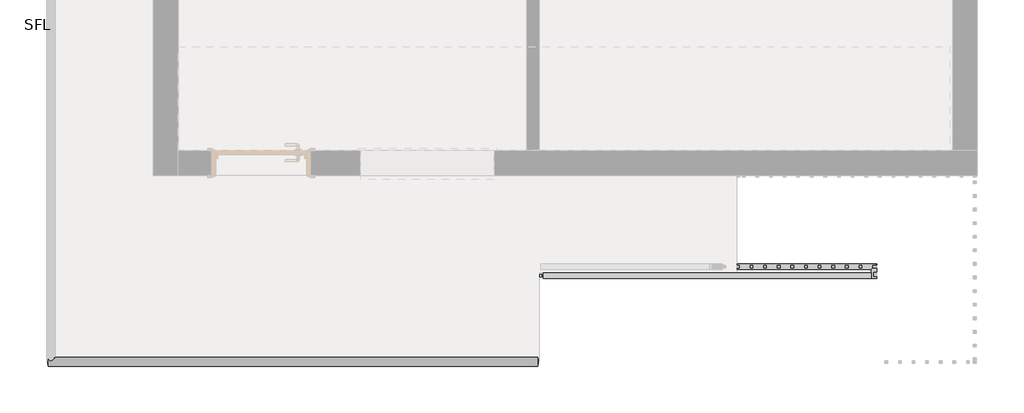
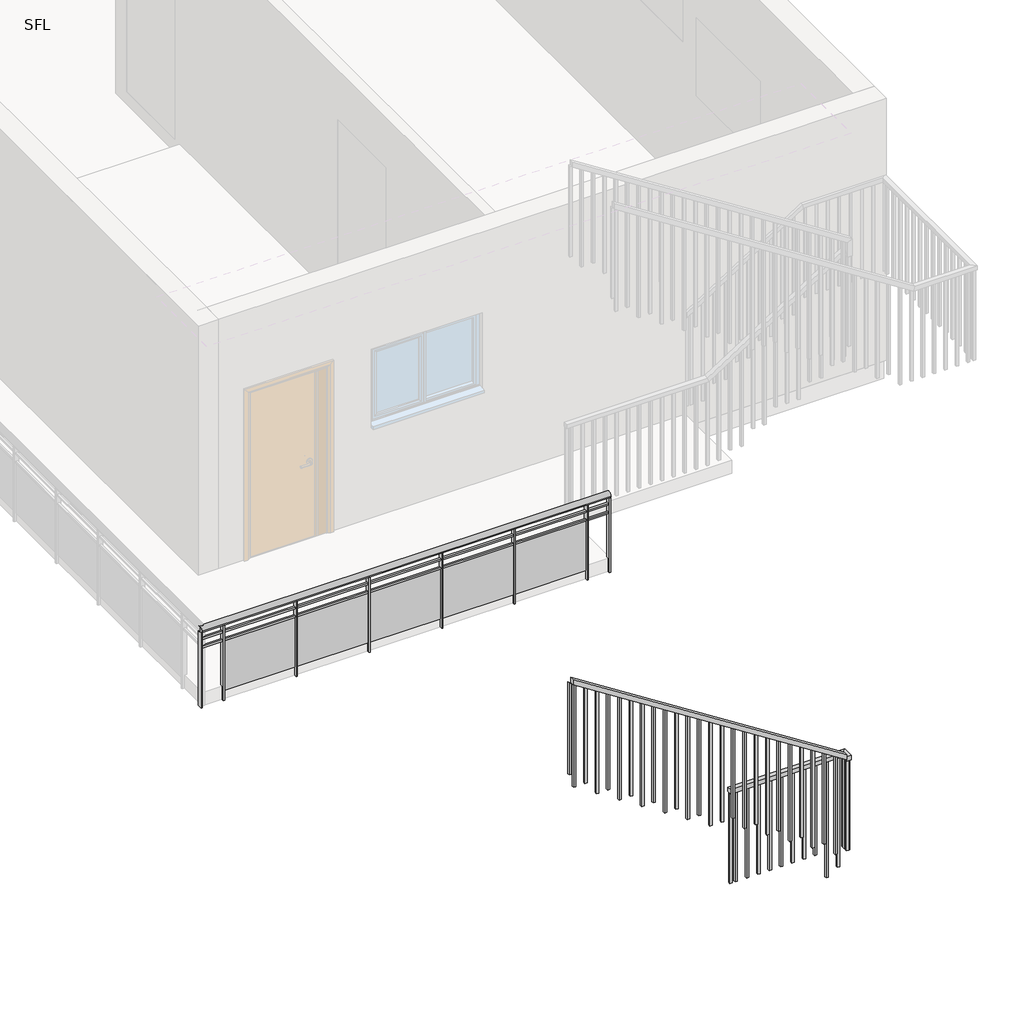
# One storey, part 2 of 4: 3 railings.
"""IFC4 building model written with IfcOpenShell, lengths in millimetres."""

from ifc_helpers import new_model, si_unit, point, frame, origin, place, context, project, spatial, polyline, ellipse_curve, trimmed, outline, extrude, faceted_brep, element, save
from ifc_brep_helpers import plane_surface, extruded_surface, advanced_brep

model = new_model("IFC4")

# Units and contexts
model_context = context("Model", 3, world=origin())
ifc_project = project(units=[si_unit("LENGTHUNIT", "METRE", prefix="MILLI")], contexts=[model_context])

# Site, building, storey
site = spatial("IfcSite", under=ifc_project)
building = spatial("IfcBuilding", under=site)
storey = spatial("IfcBuildingStorey", under=building, Name="SFL", Elevation=6583.68)

# Railings
placement = place(None, origin())
element("IfcRailing", 1, ObjectType="1100mm", at=placement, inside=storey, context=model_context, shape_type="SolidModel", body=[
    faceted_brep([(-10457.8773536, -11114.0601959, 4838.88), (-10457.8773536, -11114.0601959, 4779.5164137), (-10457.8773536, -11164.0601959, 4779.5164137), (-10457.8773536, -11164.0601959, 4838.88), (-7447.5340108, -11114.0601959, 2912.2269781), (-7447.5340108, -11164.0601959, 2912.2269781), (-7447.5340108, -11164.0601959, 2852.8633918), (-7447.5340108, -11114.0601959, 2852.8633918)], [[[0, 1, 2, 3]], [[4, 5, 6, 7]], [[1, 0, 4, 7]], [[2, 1, 7, 6]], [[3, 2, 6, 5]], [[0, 3, 5, 4]]]),
    faceted_brep([(-7447.5340108, -11164.0601959, 2888.16), (-7447.5340108, -11164.0601959, 2838.16), (-7397.5340108, -11164.0601959, 2838.16), (-7397.5340108, -11164.0601959, 2888.16), (-7447.5340108, -11083.3255223, 2888.16), (-7447.5340108, -11083.3255223, 2838.16), (-7397.5340108, -11033.3255223, 2838.16), (-7397.5340108, -11033.3255223, 2888.16), (-8680.149573, -11083.3255223, 2888.16), (-8680.149573, -11033.3255223, 2888.16), (-8680.149573, -11033.3255223, 2838.16), (-8680.149573, -11083.3255223, 2838.16)], [[[0, 1, 2, 3]], [[1, 0, 4, 5]], [[2, 1, 5, 6]], [[3, 2, 6, 7]], [[0, 3, 7, 4]], [[8, 9, 10, 11]], [[5, 4, 8, 11]], [[6, 5, 11, 10]], [[7, 6, 10, 9]], [[4, 7, 9, 8]]]),
    extrude(outline(polyline([(-8597.5340108, -11045.8255223), (-8597.5340108, -11070.8255223), (-8622.5340108, -11070.8255223), (-8622.5340108, -11045.8255223), (-8597.5340108, -11045.8255223)])), frame((0.0, 0.0, 1788.16), z_axis=(0.0, 0.0, 1.0), x_axis=(1.0, 0.0, 0.0)), (0.0, 0.0, 1.0), 1050.0),
    extrude(outline(polyline([(-8472.5340108, -11045.8255223), (-8472.5340108, -11070.8255223), (-8497.5340108, -11070.8255223), (-8497.5340108, -11045.8255223), (-8472.5340108, -11045.8255223)])), frame((0.0, 0.0, 1788.16), z_axis=(0.0, 0.0, 1.0), x_axis=(1.0, 0.0, 0.0)), (0.0, 0.0, 1.0), 1050.0),
    extrude(outline(polyline([(-8347.5340108, -11045.8255223), (-8347.5340108, -11070.8255223), (-8372.5340108, -11070.8255223), (-8372.5340108, -11045.8255223), (-8347.5340108, -11045.8255223)])), frame((0.0, 0.0, 1788.16), z_axis=(0.0, 0.0, 1.0), x_axis=(1.0, 0.0, 0.0)), (0.0, 0.0, 1.0), 1050.0),
    extrude(outline(polyline([(-8222.5340108, -11045.8255223), (-8222.5340108, -11070.8255223), (-8247.5340108, -11070.8255223), (-8247.5340108, -11045.8255223), (-8222.5340108, -11045.8255223)])), frame((0.0, 0.0, 1788.16), z_axis=(0.0, 0.0, 1.0), x_axis=(1.0, 0.0, 0.0)), (0.0, 0.0, 1.0), 1050.0),
    extrude(outline(polyline([(-8097.5340108, -11045.8255223), (-8097.5340108, -11070.8255223), (-8122.5340108, -11070.8255223), (-8122.5340108, -11045.8255223), (-8097.5340108, -11045.8255223)])), frame((0.0, 0.0, 1788.16), z_axis=(0.0, 0.0, 1.0), x_axis=(1.0, 0.0, 0.0)), (0.0, 0.0, 1.0), 1050.0),
    extrude(outline(polyline([(-7972.5340108, -11045.8255223), (-7972.5340108, -11070.8255223), (-7997.5340108, -11070.8255223), (-7997.5340108, -11045.8255223), (-7972.5340108, -11045.8255223)])), frame((0.0, 0.0, 1788.16), z_axis=(0.0, 0.0, 1.0), x_axis=(1.0, 0.0, 0.0)), (0.0, 0.0, 1.0), 1050.0),
    extrude(outline(polyline([(-7847.5340108, -11045.8255223), (-7847.5340108, -11070.8255223), (-7872.5340108, -11070.8255223), (-7872.5340108, -11045.8255223), (-7847.5340108, -11045.8255223)])), frame((0.0, 0.0, 1788.16), z_axis=(0.0, 0.0, 1.0), x_axis=(1.0, 0.0, 0.0)), (0.0, 0.0, 1.0), 1050.0),
    extrude(outline(polyline([(-7722.5340108, -11045.8255223), (-7722.5340108, -11070.8255223), (-7747.5340108, -11070.8255223), (-7747.5340108, -11045.8255223), (-7722.5340108, -11045.8255223)])), frame((0.0, 0.0, 1788.16), z_axis=(0.0, 0.0, 1.0), x_axis=(1.0, 0.0, 0.0)), (0.0, 0.0, 1.0), 1050.0),
    extrude(outline(polyline([(-7597.5340108, -11045.8255223), (-7597.5340108, -11070.8255223), (-7622.5340108, -11070.8255223), (-7622.5340108, -11045.8255223), (-7597.5340108, -11045.8255223)])), frame((0.0, 0.0, 1484.4784954), z_axis=(0.0, 0.0, 1.0), x_axis=(1.0, 0.0, 0.0)), (0.0, 0.0, 1.0), 1353.6815046),
    extrude(outline(polyline([(-7472.5340108, -11045.8255223), (-7472.5340108, -11070.8255223), (-7497.5340108, -11070.8255223), (-7497.5340108, -11045.8255223), (-7472.5340108, -11045.8255223)])), frame((0.0, 0.0, 1564.4608651), z_axis=(0.0, 0.0, 1.0), x_axis=(1.0, 0.0, 0.0)), (0.0, 0.0, 1.0), 1273.6991349),
    extrude(outline(polyline([(-7410.0340108, -11089.0601959), (-7435.0340108, -11089.0601959), (-7435.0340108, -11064.0601959), (-7410.0340108, -11064.0601959), (-7410.0340108, -11089.0601959)])), frame((0.0, 0.0, 1770.6), z_axis=(0.0, 0.0, 1.0), x_axis=(1.0, 0.0, 0.0)), (0.0, 0.0, 1.0), 1067.56),
    extrude(outline(polyline([(2851.8393741, -7445.9340108), (1788.16, -7445.9340108), (1788.16, -7420.9340108), (2835.8390977, -7420.9340108), (2851.8393741, -7445.9340108)])), frame((0.0, -11151.5601959, 0.0), z_axis=(0.0, 1.0, 0.0), x_axis=(0.0, 0.0, 1.0)), (0.0, 0.0, 1.0), 25.0),
    extrude(outline(polyline([(2931.8407561, -7570.9340108), (1788.16, -7570.9340108), (1788.16, -7545.9340108), (2915.8404797, -7545.9340108), (2931.8407561, -7570.9340108)])), frame((0.0, -11151.5601959, 0.0), z_axis=(0.0, 1.0, 0.0), x_axis=(0.0, 0.0, 1.0)), (0.0, 0.0, 1.0), 25.0),
    extrude(outline(polyline([(3011.8421381, -7695.9340108), (1950.72, -7695.9340108), (1950.72, -7670.9340108), (2995.8418617, -7670.9340108), (3011.8421381, -7695.9340108)])), frame((0.0, -11151.5601959, 0.0), z_axis=(0.0, 1.0, 0.0), x_axis=(0.0, 0.0, 1.0)), (0.0, 0.0, 1.0), 25.0),
    extrude(outline(polyline([(3091.8435201, -7820.9340108), (1950.72, -7820.9340108), (1950.72, -7795.9340108), (3075.8432437, -7795.9340108), (3091.8435201, -7820.9340108)])), frame((0.0, -11151.5601959, 0.0), z_axis=(0.0, 1.0, 0.0), x_axis=(0.0, 0.0, 1.0)), (0.0, 0.0, 1.0), 25.0),
    extrude(outline(polyline([(3171.8449021, -7945.9340108), (2113.28, -7945.9340108), (2113.28, -7920.9340108), (3155.8446257, -7920.9340108), (3171.8449021, -7945.9340108)])), frame((0.0, -11151.5601959, 0.0), z_axis=(0.0, 1.0, 0.0), x_axis=(0.0, 0.0, 1.0)), (0.0, 0.0, 1.0), 25.0),
    extrude(outline(polyline([(3251.8462841, -8070.9340108), (2113.28, -8070.9340108), (2113.28, -8045.9340108), (3235.8460077, -8045.9340108), (3251.8462841, -8070.9340108)])), frame((0.0, -11151.5601959, 0.0), z_axis=(0.0, 1.0, 0.0), x_axis=(0.0, 0.0, 1.0)), (0.0, 0.0, 1.0), 25.0),
    extrude(outline(polyline([(3331.8476661, -8195.9340108), (2275.84, -8195.9340108), (2275.84, -8170.9340108), (3315.8473897, -8170.9340108), (3331.8476661, -8195.9340108)])), frame((0.0, -11151.5601959, 0.0), z_axis=(0.0, 1.0, 0.0), x_axis=(0.0, 0.0, 1.0)), (0.0, 0.0, 1.0), 25.0),
    extrude(outline(polyline([(3411.8490481, -8320.9340108), (2275.84, -8320.9340108), (2275.84, -8295.9340108), (3395.8487717, -8295.9340108), (3411.8490481, -8320.9340108)])), frame((0.0, -11151.5601959, 0.0), z_axis=(0.0, 1.0, 0.0), x_axis=(0.0, 0.0, 1.0)), (0.0, 0.0, 1.0), 25.0),
    extrude(outline(polyline([(3491.8504301, -8445.9340108), (2438.4, -8445.9340108), (2438.4, -8420.9340108), (3475.8501537, -8420.9340108), (3491.8504301, -8445.9340108)])), frame((0.0, -11151.5601959, 0.0), z_axis=(0.0, 1.0, 0.0), x_axis=(0.0, 0.0, 1.0)), (0.0, 0.0, 1.0), 25.0),
    extrude(outline(polyline([(3571.8518121, -8570.9340108), (2438.4, -8570.9340108), (2438.4, -8545.9340108), (3555.8515357, -8545.9340108), (3571.8518121, -8570.9340108)])), frame((0.0, -11151.5601959, 0.0), z_axis=(0.0, 1.0, 0.0), x_axis=(0.0, 0.0, 1.0)), (0.0, 0.0, 1.0), 25.0),
    extrude(outline(polyline([(3651.8531942, -8695.9340108), (2600.96, -8695.9340108), (2600.96, -8670.9340108), (3635.8529178, -8670.9340108), (3651.8531942, -8695.9340108)])), frame((0.0, -11151.5601959, 0.0), z_axis=(0.0, 1.0, 0.0), x_axis=(0.0, 0.0, 1.0)), (0.0, 0.0, 1.0), 25.0),
    extrude(outline(polyline([(3731.8545762, -8820.9340108), (2600.96, -8820.9340108), (2600.96, -8795.9340108), (3715.8542998, -8795.9340108), (3731.8545762, -8820.9340108)])), frame((0.0, -11151.5601959, 0.0), z_axis=(0.0, 1.0, 0.0), x_axis=(0.0, 0.0, 1.0)), (0.0, 0.0, 1.0), 25.0),
    extrude(outline(polyline([(3811.8559582, -8945.9340108), (2600.96, -8945.9340108), (2600.96, -8920.9340108), (3795.8556818, -8920.9340108), (3811.8559582, -8945.9340108)])), frame((0.0, -11151.5601959, 0.0), z_axis=(0.0, 1.0, 0.0), x_axis=(0.0, 0.0, 1.0)), (0.0, 0.0, 1.0), 25.0),
    extrude(outline(polyline([(3891.8573402, -9070.9340108), (2763.52, -9070.9340108), (2763.52, -9045.9340108), (3875.8570638, -9045.9340108), (3891.8573402, -9070.9340108)])), frame((0.0, -11151.5601959, 0.0), z_axis=(0.0, 1.0, 0.0), x_axis=(0.0, 0.0, 1.0)), (0.0, 0.0, 1.0), 25.0),
    extrude(outline(polyline([(3971.8587222, -9195.9340108), (2763.52, -9195.9340108), (2763.52, -9170.9340108), (3955.8584458, -9170.9340108), (3971.8587222, -9195.9340108)])), frame((0.0, -11151.5601959, 0.0), z_axis=(0.0, 1.0, 0.0), x_axis=(0.0, 0.0, 1.0)), (0.0, 0.0, 1.0), 25.0),
    extrude(outline(polyline([(4051.8601042, -9320.9340108), (2926.08, -9320.9340108), (2926.08, -9295.9340108), (4035.8598278, -9295.9340108), (4051.8601042, -9320.9340108)])), frame((0.0, -11151.5601959, 0.0), z_axis=(0.0, 1.0, 0.0), x_axis=(0.0, 0.0, 1.0)), (0.0, 0.0, 1.0), 25.0),
    extrude(outline(polyline([(4131.8614862, -9445.9340108), (2926.08, -9445.9340108), (2926.08, -9420.9340108), (4115.8612098, -9420.9340108), (4131.8614862, -9445.9340108)])), frame((0.0, -11151.5601959, 0.0), z_axis=(0.0, 1.0, 0.0), x_axis=(0.0, 0.0, 1.0)), (0.0, 0.0, 1.0), 25.0),
    extrude(outline(polyline([(4211.8628682, -9570.9340108), (3088.64, -9570.9340108), (3088.64, -9545.9340108), (4195.8625918, -9545.9340108), (4211.8628682, -9570.9340108)])), frame((0.0, -11151.5601959, 0.0), z_axis=(0.0, 1.0, 0.0), x_axis=(0.0, 0.0, 1.0)), (0.0, 0.0, 1.0), 25.0),
    extrude(outline(polyline([(4291.8642502, -9695.9340108), (3088.64, -9695.9340108), (3088.64, -9670.9340108), (4275.8639738, -9670.9340108), (4291.8642502, -9695.9340108)])), frame((0.0, -11151.5601959, 0.0), z_axis=(0.0, 1.0, 0.0), x_axis=(0.0, 0.0, 1.0)), (0.0, 0.0, 1.0), 25.0),
    extrude(outline(polyline([(4371.8656322, -9820.9340108), (3251.2, -9820.9340108), (3251.2, -9795.9340108), (4355.8653558, -9795.9340108), (4371.8656322, -9820.9340108)])), frame((0.0, -11151.5601959, 0.0), z_axis=(0.0, 1.0, 0.0), x_axis=(0.0, 0.0, 1.0)), (0.0, 0.0, 1.0), 25.0),
    extrude(outline(polyline([(4451.8670143, -9945.9340108), (3251.2, -9945.9340108), (3251.2, -9920.9340108), (4435.8667379, -9920.9340108), (4451.8670143, -9945.9340108)])), frame((0.0, -11151.5601959, 0.0), z_axis=(0.0, 1.0, 0.0), x_axis=(0.0, 0.0, 1.0)), (0.0, 0.0, 1.0), 25.0),
    extrude(outline(polyline([(4531.8683963, -10070.9340108), (3413.76, -10070.9340108), (3413.76, -10045.9340108), (4515.8681199, -10045.9340108), (4531.8683963, -10070.9340108)])), frame((0.0, -11151.5601959, 0.0), z_axis=(0.0, 1.0, 0.0), x_axis=(0.0, 0.0, 1.0)), (0.0, 0.0, 1.0), 25.0),
    extrude(outline(polyline([(4611.8697783, -10195.9340108), (3413.76, -10195.9340108), (3413.76, -10170.9340108), (4595.8695019, -10170.9340108), (4611.8697783, -10195.9340108)])), frame((0.0, -11151.5601959, 0.0), z_axis=(0.0, 1.0, 0.0), x_axis=(0.0, 0.0, 1.0)), (0.0, 0.0, 1.0), 25.0),
    extrude(outline(polyline([(4691.8711603, -10320.9340108), (3576.32, -10320.9340108), (3576.32, -10295.9340108), (4675.8708839, -10295.9340108), (4691.8711603, -10320.9340108)])), frame((0.0, -11151.5601959, 0.0), z_axis=(0.0, 1.0, 0.0), x_axis=(0.0, 0.0, 1.0)), (0.0, 0.0, 1.0), 25.0),
    extrude(outline(polyline([(4771.8725423, -10445.9340108), (3576.32, -10445.9340108), (3576.32, -10420.9340108), (4755.8722659, -10420.9340108), (4771.8725423, -10445.9340108)])), frame((0.0, -11151.5601959, 0.0), z_axis=(0.0, 1.0, 0.0), x_axis=(0.0, 0.0, 1.0)), (0.0, 0.0, 1.0), 25.0),
    extrude(outline(polyline([(-7410.0340108, -11070.8255223), (-7435.0340108, -11070.8255223), (-7435.0340108, -11045.8255223), (-7410.0340108, -11045.8255223), (-7410.0340108, -11070.8255223)])), frame((0.0, 0.0, 1770.6), z_axis=(0.0, 0.0, 1.0), x_axis=(1.0, 0.0, 0.0)), (0.0, 0.0, 1.0), 1067.56),
    extrude(outline(polyline([(2844.8632536, -7435.0340108), (1788.16, -7435.0340108), (1788.16, -7410.0340108), (2828.8629772, -7410.0340108), (2844.8632536, -7435.0340108)])), frame((0.0, -11151.5601959, 0.0), z_axis=(0.0, 1.0, 0.0), x_axis=(0.0, 0.0, 1.0)), (0.0, 0.0, 1.0), 25.0),
    extrude(outline(polyline([(-8655.149573, -11045.8255223), (-8655.149573, -11070.8255223), (-8680.149573, -11070.8255223), (-8680.149573, -11045.8255223), (-8655.149573, -11045.8255223)])), frame((0.0, 0.0, 1788.16), z_axis=(0.0, 0.0, 1.0), x_axis=(1.0, 0.0, 0.0)), (0.0, 0.0, 1.0), 1050.0),
    extrude(outline(polyline([(4803.8730951, -10495.9340108), (3738.88, -10495.9340108), (3738.88, -10470.9340108), (4787.8728187, -10470.9340108), (4803.8730951, -10495.9340108)])), frame((0.0, -11151.5601959, 0.0), z_axis=(0.0, 1.0, 0.0), x_axis=(0.0, 0.0, 1.0)), (0.0, 0.0, 1.0), 25.0),
])
element("IfcRailing", 2, ObjectType="1100mm", at=placement, inside=storey, context=model_context, shape_type="SolidModel", body=[
    faceted_brep([(-10457.8773536, -11114.0601959, 4838.88), (-10457.8773536, -11114.0601959, 4779.5164137), (-10457.8773536, -11164.0601959, 4779.5164137), (-10457.8773536, -11164.0601959, 4838.88), (-7447.5340108, -11114.0601959, 2912.2269781), (-7447.5340108, -11164.0601959, 2912.2269781), (-7447.5340108, -11164.0601959, 2852.8633918), (-7447.5340108, -11114.0601959, 2852.8633918)], [[[0, 1, 2, 3]], [[4, 5, 6, 7]], [[1, 0, 4, 7]], [[2, 1, 7, 6]], [[3, 2, 6, 5]], [[0, 3, 5, 4]]]),
    faceted_brep([(-7447.5340108, -11164.0601959, 2888.16), (-7447.5340108, -11164.0601959, 2838.16), (-7397.5340108, -11164.0601959, 2838.16), (-7397.5340108, -11164.0601959, 2888.16), (-7447.5340108, -11083.3255223, 2888.16), (-7447.5340108, -11083.3255223, 2838.16), (-7397.5340108, -11033.3255223, 2838.16), (-7397.5340108, -11033.3255223, 2888.16), (-8680.149573, -11083.3255223, 2888.16), (-8680.149573, -11033.3255223, 2888.16), (-8680.149573, -11033.3255223, 2838.16), (-8680.149573, -11083.3255223, 2838.16)], [[[0, 1, 2, 3]], [[1, 0, 4, 5]], [[2, 1, 5, 6]], [[3, 2, 6, 7]], [[0, 3, 7, 4]], [[8, 9, 10, 11]], [[5, 4, 8, 11]], [[6, 5, 11, 10]], [[7, 6, 10, 9]], [[4, 7, 9, 8]]]),
    extrude(outline(polyline([(-8597.5340108, -11045.8255223), (-8597.5340108, -11070.8255223), (-8622.5340108, -11070.8255223), (-8622.5340108, -11045.8255223), (-8597.5340108, -11045.8255223)])), frame((0.0, 0.0, 1788.16), z_axis=(0.0, 0.0, 1.0), x_axis=(1.0, 0.0, 0.0)), (0.0, 0.0, 1.0), 1050.0),
    extrude(outline(polyline([(-8472.5340108, -11045.8255223), (-8472.5340108, -11070.8255223), (-8497.5340108, -11070.8255223), (-8497.5340108, -11045.8255223), (-8472.5340108, -11045.8255223)])), frame((0.0, 0.0, 1788.16), z_axis=(0.0, 0.0, 1.0), x_axis=(1.0, 0.0, 0.0)), (0.0, 0.0, 1.0), 1050.0),
    extrude(outline(polyline([(-8347.5340108, -11045.8255223), (-8347.5340108, -11070.8255223), (-8372.5340108, -11070.8255223), (-8372.5340108, -11045.8255223), (-8347.5340108, -11045.8255223)])), frame((0.0, 0.0, 1788.16), z_axis=(0.0, 0.0, 1.0), x_axis=(1.0, 0.0, 0.0)), (0.0, 0.0, 1.0), 1050.0),
    extrude(outline(polyline([(-8222.5340108, -11045.8255223), (-8222.5340108, -11070.8255223), (-8247.5340108, -11070.8255223), (-8247.5340108, -11045.8255223), (-8222.5340108, -11045.8255223)])), frame((0.0, 0.0, 1788.16), z_axis=(0.0, 0.0, 1.0), x_axis=(1.0, 0.0, 0.0)), (0.0, 0.0, 1.0), 1050.0),
    extrude(outline(polyline([(-8097.5340108, -11045.8255223), (-8097.5340108, -11070.8255223), (-8122.5340108, -11070.8255223), (-8122.5340108, -11045.8255223), (-8097.5340108, -11045.8255223)])), frame((0.0, 0.0, 1788.16), z_axis=(0.0, 0.0, 1.0), x_axis=(1.0, 0.0, 0.0)), (0.0, 0.0, 1.0), 1050.0),
    extrude(outline(polyline([(-7972.5340108, -11045.8255223), (-7972.5340108, -11070.8255223), (-7997.5340108, -11070.8255223), (-7997.5340108, -11045.8255223), (-7972.5340108, -11045.8255223)])), frame((0.0, 0.0, 1788.16), z_axis=(0.0, 0.0, 1.0), x_axis=(1.0, 0.0, 0.0)), (0.0, 0.0, 1.0), 1050.0),
    extrude(outline(polyline([(-7847.5340108, -11045.8255223), (-7847.5340108, -11070.8255223), (-7872.5340108, -11070.8255223), (-7872.5340108, -11045.8255223), (-7847.5340108, -11045.8255223)])), frame((0.0, 0.0, 1788.16), z_axis=(0.0, 0.0, 1.0), x_axis=(1.0, 0.0, 0.0)), (0.0, 0.0, 1.0), 1050.0),
    extrude(outline(polyline([(-7722.5340108, -11045.8255223), (-7722.5340108, -11070.8255223), (-7747.5340108, -11070.8255223), (-7747.5340108, -11045.8255223), (-7722.5340108, -11045.8255223)])), frame((0.0, 0.0, 1788.16), z_axis=(0.0, 0.0, 1.0), x_axis=(1.0, 0.0, 0.0)), (0.0, 0.0, 1.0), 1050.0),
    extrude(outline(polyline([(-7597.5340108, -11045.8255223), (-7597.5340108, -11070.8255223), (-7622.5340108, -11070.8255223), (-7622.5340108, -11045.8255223), (-7597.5340108, -11045.8255223)])), frame((0.0, 0.0, 1484.4784954), z_axis=(0.0, 0.0, 1.0), x_axis=(1.0, 0.0, 0.0)), (0.0, 0.0, 1.0), 1353.6815046),
    extrude(outline(polyline([(-7472.5340108, -11045.8255223), (-7472.5340108, -11070.8255223), (-7497.5340108, -11070.8255223), (-7497.5340108, -11045.8255223), (-7472.5340108, -11045.8255223)])), frame((0.0, 0.0, 1564.4608651), z_axis=(0.0, 0.0, 1.0), x_axis=(1.0, 0.0, 0.0)), (0.0, 0.0, 1.0), 1273.6991349),
    extrude(outline(polyline([(-7410.0340108, -11089.0601959), (-7435.0340108, -11089.0601959), (-7435.0340108, -11064.0601959), (-7410.0340108, -11064.0601959), (-7410.0340108, -11089.0601959)])), frame((0.0, 0.0, 1770.6), z_axis=(0.0, 0.0, 1.0), x_axis=(1.0, 0.0, 0.0)), (0.0, 0.0, 1.0), 1067.56),
    extrude(outline(polyline([(2851.8393741, -7445.9340108), (1788.16, -7445.9340108), (1788.16, -7420.9340108), (2835.8390977, -7420.9340108), (2851.8393741, -7445.9340108)])), frame((0.0, -11151.5601959, 0.0), z_axis=(0.0, 1.0, 0.0), x_axis=(0.0, 0.0, 1.0)), (0.0, 0.0, 1.0), 25.0),
    extrude(outline(polyline([(2931.8407561, -7570.9340108), (1788.16, -7570.9340108), (1788.16, -7545.9340108), (2915.8404797, -7545.9340108), (2931.8407561, -7570.9340108)])), frame((0.0, -11151.5601959, 0.0), z_axis=(0.0, 1.0, 0.0), x_axis=(0.0, 0.0, 1.0)), (0.0, 0.0, 1.0), 25.0),
    extrude(outline(polyline([(3011.8421381, -7695.9340108), (1950.72, -7695.9340108), (1950.72, -7670.9340108), (2995.8418617, -7670.9340108), (3011.8421381, -7695.9340108)])), frame((0.0, -11151.5601959, 0.0), z_axis=(0.0, 1.0, 0.0), x_axis=(0.0, 0.0, 1.0)), (0.0, 0.0, 1.0), 25.0),
    extrude(outline(polyline([(3091.8435201, -7820.9340108), (1950.72, -7820.9340108), (1950.72, -7795.9340108), (3075.8432437, -7795.9340108), (3091.8435201, -7820.9340108)])), frame((0.0, -11151.5601959, 0.0), z_axis=(0.0, 1.0, 0.0), x_axis=(0.0, 0.0, 1.0)), (0.0, 0.0, 1.0), 25.0),
    extrude(outline(polyline([(3171.8449021, -7945.9340108), (2113.28, -7945.9340108), (2113.28, -7920.9340108), (3155.8446257, -7920.9340108), (3171.8449021, -7945.9340108)])), frame((0.0, -11151.5601959, 0.0), z_axis=(0.0, 1.0, 0.0), x_axis=(0.0, 0.0, 1.0)), (0.0, 0.0, 1.0), 25.0),
    extrude(outline(polyline([(3251.8462841, -8070.9340108), (2113.28, -8070.9340108), (2113.28, -8045.9340108), (3235.8460077, -8045.9340108), (3251.8462841, -8070.9340108)])), frame((0.0, -11151.5601959, 0.0), z_axis=(0.0, 1.0, 0.0), x_axis=(0.0, 0.0, 1.0)), (0.0, 0.0, 1.0), 25.0),
    extrude(outline(polyline([(3331.8476661, -8195.9340108), (2275.84, -8195.9340108), (2275.84, -8170.9340108), (3315.8473897, -8170.9340108), (3331.8476661, -8195.9340108)])), frame((0.0, -11151.5601959, 0.0), z_axis=(0.0, 1.0, 0.0), x_axis=(0.0, 0.0, 1.0)), (0.0, 0.0, 1.0), 25.0),
    extrude(outline(polyline([(3411.8490481, -8320.9340108), (2275.84, -8320.9340108), (2275.84, -8295.9340108), (3395.8487717, -8295.9340108), (3411.8490481, -8320.9340108)])), frame((0.0, -11151.5601959, 0.0), z_axis=(0.0, 1.0, 0.0), x_axis=(0.0, 0.0, 1.0)), (0.0, 0.0, 1.0), 25.0),
    extrude(outline(polyline([(3491.8504301, -8445.9340108), (2438.4, -8445.9340108), (2438.4, -8420.9340108), (3475.8501537, -8420.9340108), (3491.8504301, -8445.9340108)])), frame((0.0, -11151.5601959, 0.0), z_axis=(0.0, 1.0, 0.0), x_axis=(0.0, 0.0, 1.0)), (0.0, 0.0, 1.0), 25.0),
    extrude(outline(polyline([(3571.8518121, -8570.9340108), (2438.4, -8570.9340108), (2438.4, -8545.9340108), (3555.8515357, -8545.9340108), (3571.8518121, -8570.9340108)])), frame((0.0, -11151.5601959, 0.0), z_axis=(0.0, 1.0, 0.0), x_axis=(0.0, 0.0, 1.0)), (0.0, 0.0, 1.0), 25.0),
    extrude(outline(polyline([(3651.8531942, -8695.9340108), (2600.96, -8695.9340108), (2600.96, -8670.9340108), (3635.8529178, -8670.9340108), (3651.8531942, -8695.9340108)])), frame((0.0, -11151.5601959, 0.0), z_axis=(0.0, 1.0, 0.0), x_axis=(0.0, 0.0, 1.0)), (0.0, 0.0, 1.0), 25.0),
    extrude(outline(polyline([(3731.8545762, -8820.9340108), (2600.96, -8820.9340108), (2600.96, -8795.9340108), (3715.8542998, -8795.9340108), (3731.8545762, -8820.9340108)])), frame((0.0, -11151.5601959, 0.0), z_axis=(0.0, 1.0, 0.0), x_axis=(0.0, 0.0, 1.0)), (0.0, 0.0, 1.0), 25.0),
    extrude(outline(polyline([(3811.8559582, -8945.9340108), (2600.96, -8945.9340108), (2600.96, -8920.9340108), (3795.8556818, -8920.9340108), (3811.8559582, -8945.9340108)])), frame((0.0, -11151.5601959, 0.0), z_axis=(0.0, 1.0, 0.0), x_axis=(0.0, 0.0, 1.0)), (0.0, 0.0, 1.0), 25.0),
    extrude(outline(polyline([(3891.8573402, -9070.9340108), (2763.52, -9070.9340108), (2763.52, -9045.9340108), (3875.8570638, -9045.9340108), (3891.8573402, -9070.9340108)])), frame((0.0, -11151.5601959, 0.0), z_axis=(0.0, 1.0, 0.0), x_axis=(0.0, 0.0, 1.0)), (0.0, 0.0, 1.0), 25.0),
    extrude(outline(polyline([(3971.8587222, -9195.9340108), (2763.52, -9195.9340108), (2763.52, -9170.9340108), (3955.8584458, -9170.9340108), (3971.8587222, -9195.9340108)])), frame((0.0, -11151.5601959, 0.0), z_axis=(0.0, 1.0, 0.0), x_axis=(0.0, 0.0, 1.0)), (0.0, 0.0, 1.0), 25.0),
    extrude(outline(polyline([(4051.8601042, -9320.9340108), (2926.08, -9320.9340108), (2926.08, -9295.9340108), (4035.8598278, -9295.9340108), (4051.8601042, -9320.9340108)])), frame((0.0, -11151.5601959, 0.0), z_axis=(0.0, 1.0, 0.0), x_axis=(0.0, 0.0, 1.0)), (0.0, 0.0, 1.0), 25.0),
    extrude(outline(polyline([(4131.8614862, -9445.9340108), (2926.08, -9445.9340108), (2926.08, -9420.9340108), (4115.8612098, -9420.9340108), (4131.8614862, -9445.9340108)])), frame((0.0, -11151.5601959, 0.0), z_axis=(0.0, 1.0, 0.0), x_axis=(0.0, 0.0, 1.0)), (0.0, 0.0, 1.0), 25.0),
    extrude(outline(polyline([(4211.8628682, -9570.9340108), (3088.64, -9570.9340108), (3088.64, -9545.9340108), (4195.8625918, -9545.9340108), (4211.8628682, -9570.9340108)])), frame((0.0, -11151.5601959, 0.0), z_axis=(0.0, 1.0, 0.0), x_axis=(0.0, 0.0, 1.0)), (0.0, 0.0, 1.0), 25.0),
    extrude(outline(polyline([(4291.8642502, -9695.9340108), (3088.64, -9695.9340108), (3088.64, -9670.9340108), (4275.8639738, -9670.9340108), (4291.8642502, -9695.9340108)])), frame((0.0, -11151.5601959, 0.0), z_axis=(0.0, 1.0, 0.0), x_axis=(0.0, 0.0, 1.0)), (0.0, 0.0, 1.0), 25.0),
    extrude(outline(polyline([(4371.8656322, -9820.9340108), (3251.2, -9820.9340108), (3251.2, -9795.9340108), (4355.8653558, -9795.9340108), (4371.8656322, -9820.9340108)])), frame((0.0, -11151.5601959, 0.0), z_axis=(0.0, 1.0, 0.0), x_axis=(0.0, 0.0, 1.0)), (0.0, 0.0, 1.0), 25.0),
    extrude(outline(polyline([(4451.8670143, -9945.9340108), (3251.2, -9945.9340108), (3251.2, -9920.9340108), (4435.8667379, -9920.9340108), (4451.8670143, -9945.9340108)])), frame((0.0, -11151.5601959, 0.0), z_axis=(0.0, 1.0, 0.0), x_axis=(0.0, 0.0, 1.0)), (0.0, 0.0, 1.0), 25.0),
    extrude(outline(polyline([(4531.8683963, -10070.9340108), (3413.76, -10070.9340108), (3413.76, -10045.9340108), (4515.8681199, -10045.9340108), (4531.8683963, -10070.9340108)])), frame((0.0, -11151.5601959, 0.0), z_axis=(0.0, 1.0, 0.0), x_axis=(0.0, 0.0, 1.0)), (0.0, 0.0, 1.0), 25.0),
    extrude(outline(polyline([(4611.8697783, -10195.9340108), (3413.76, -10195.9340108), (3413.76, -10170.9340108), (4595.8695019, -10170.9340108), (4611.8697783, -10195.9340108)])), frame((0.0, -11151.5601959, 0.0), z_axis=(0.0, 1.0, 0.0), x_axis=(0.0, 0.0, 1.0)), (0.0, 0.0, 1.0), 25.0),
    extrude(outline(polyline([(4691.8711603, -10320.9340108), (3576.32, -10320.9340108), (3576.32, -10295.9340108), (4675.8708839, -10295.9340108), (4691.8711603, -10320.9340108)])), frame((0.0, -11151.5601959, 0.0), z_axis=(0.0, 1.0, 0.0), x_axis=(0.0, 0.0, 1.0)), (0.0, 0.0, 1.0), 25.0),
    extrude(outline(polyline([(4771.8725423, -10445.9340108), (3576.32, -10445.9340108), (3576.32, -10420.9340108), (4755.8722659, -10420.9340108), (4771.8725423, -10445.9340108)])), frame((0.0, -11151.5601959, 0.0), z_axis=(0.0, 1.0, 0.0), x_axis=(0.0, 0.0, 1.0)), (0.0, 0.0, 1.0), 25.0),
    extrude(outline(polyline([(-7410.0340108, -11070.8255223), (-7435.0340108, -11070.8255223), (-7435.0340108, -11045.8255223), (-7410.0340108, -11045.8255223), (-7410.0340108, -11070.8255223)])), frame((0.0, 0.0, 1770.6), z_axis=(0.0, 0.0, 1.0), x_axis=(1.0, 0.0, 0.0)), (0.0, 0.0, 1.0), 1067.56),
    extrude(outline(polyline([(2844.8632536, -7435.0340108), (1788.16, -7435.0340108), (1788.16, -7410.0340108), (2828.8629772, -7410.0340108), (2844.8632536, -7435.0340108)])), frame((0.0, -11151.5601959, 0.0), z_axis=(0.0, 1.0, 0.0), x_axis=(0.0, 0.0, 1.0)), (0.0, 0.0, 1.0), 25.0),
    extrude(outline(polyline([(-8655.149573, -11045.8255223), (-8655.149573, -11070.8255223), (-8680.149573, -11070.8255223), (-8680.149573, -11045.8255223), (-8655.149573, -11045.8255223)])), frame((0.0, 0.0, 1788.16), z_axis=(0.0, 0.0, 1.0), x_axis=(1.0, 0.0, 0.0)), (0.0, 0.0, 1.0), 1050.0),
    extrude(outline(polyline([(4803.8730951, -10495.9340108), (3738.88, -10495.9340108), (3738.88, -10470.9340108), (4787.8728187, -10470.9340108), (4803.8730951, -10495.9340108)])), frame((0.0, -11151.5601959, 0.0), z_axis=(0.0, 1.0, 0.0), x_axis=(0.0, 0.0, 1.0)), (0.0, 0.0, 1.0), 25.0),
])
element("IfcRailing", 3, ObjectType="Glass_Panel-Bottom_Fill", at=placement, inside=storey, context=model_context, shape_type="SolidModel", body=[
    advanced_brep(
    [(-15004.3420435, -11892.802126, 7483.68), (-15004.3420435, -11972.802126, 7483.68), (-10508.5420435, -11892.802126, 7483.68), (-10508.5420435, -11972.802126, 7483.68)],
    [
        (0, 1, ellipse_curve(frame((-15004.3420435, -11932.802126, 7483.68), z_axis=(-1.0, 0.0, 0.0), x_axis=(0.0, -1.0, 0.0)), 40.0, 30.0)),
        (1, 0, ellipse_curve(frame((-15004.3420435, -11932.802126, 7483.68), z_axis=(-1.0, 0.0, 0.0), x_axis=(0.0, -1.0, 0.0)), 40.0, 30.0)),
        (2, 3, ellipse_curve(frame((-10508.5420435, -11932.802126, 7483.68), z_axis=(1.0, 0.0, 0.0), x_axis=(0.0, -1.0, 0.0)), 40.0, 30.0)),
        (3, 2, ellipse_curve(frame((-10508.5420435, -11932.802126, 7483.68), z_axis=(1.0, 0.0, 0.0), x_axis=(0.0, -1.0, 0.0)), 40.0, 30.0)),
        (0, 2),
        (3, 1),
    ],
    [
        plane_surface(frame((-15004.3420435, -11932.802126, 7483.68), z_axis=(-1.0, 0.0, 0.0), x_axis=(0.0, 1.0, 0.0))),
        plane_surface(frame((-10508.5420435, -11932.802126, 7483.68), z_axis=(1.0, 0.0, 0.0), x_axis=(0.0, 1.0, 0.0))),
        extruded_surface(trimmed(ellipse_curve(frame((-10508.5420435, -11932.802126, 7483.68), z_axis=(-1.0, 0.0, 0.0), x_axis=(0.0, -1.0, 0.0)), 40.0, 30.0), [point((-10508.5420435, -11892.802126, 7483.68))], [point((-10508.5420435, -11972.802126, 7483.68))], True, "CARTESIAN"), (-4495.800000000001, 0.0, 0.0), 4495.800000000001),
        extruded_surface(trimmed(ellipse_curve(frame((-10508.5420435, -11932.802126, 7483.68), z_axis=(-1.0, 0.0, 0.0), x_axis=(0.0, -1.0, 0.0)), 40.0, 30.0), [point((-10508.5420435, -11972.802126, 7483.68))], [point((-10508.5420435, -11892.802126, 7483.68))], True, "CARTESIAN"), (-4495.800000000001, 0.0, 0.0), 4495.800000000001),
    ],
    [
        (0, [[1, 2]]),
        (1, [[3, 4]]),
        (2, [[-1, 5, -4, 6]]),
        (3, [[-2, -6, -3, -5]]),
    ],
),
    extrude(outline(polyline([(-15004.3420435, -11942.1928911), (-15004.3420435, -11922.1928911), (-10508.5420435, -11922.1928911), (-10508.5420435, -11942.1928911), (-15004.3420435, -11942.1928911)])), frame((0.0, 0.0, 7363.68), z_axis=(0.0, 0.0, 1.0), x_axis=(1.0, 0.0, 0.0)), (0.0, 0.0, 1.0), 20.0),
    extrude(outline(polyline([(-15004.3420435, -11942.1928911), (-15004.3420435, -11922.1928911), (-10508.5420435, -11922.1928911), (-10508.5420435, -11942.1928911), (-15004.3420435, -11942.1928911)])), frame((0.0, 0.0, 7263.68), z_axis=(0.0, 0.0, 1.0), x_axis=(1.0, 0.0, 0.0)), (0.0, 0.0, 1.0), 20.0),
    extrude(outline(polyline([(-10762.4420435, -11907.1928911), (-10750.4420435, -11907.1928911), (-10750.4420435, -11957.1928911), (-10762.4420435, -11957.1928911), (-10762.4420435, -11907.1928911)])), frame((0.0, 0.0, 6583.68), z_axis=(0.0, 0.0, 1.0), x_axis=(1.0, 0.0, 0.0)), (0.0, 0.0, 1.0), 870.0),
    extrude(outline(polyline([(-11556.4420435, -11933.9177012), (-10756.4420435, -11933.9177012), (-10756.4420435, -11938.9177012), (-11556.4420435, -11938.9177012), (-11556.4420435, -11933.9177012)])), frame((0.0, 0.0, 6683.68), z_axis=(0.0, 0.0, 1.0), x_axis=(1.0, 0.0, 0.0)), (0.0, 0.0, 1.0), 580.0),
    extrude(outline(polyline([(-11562.4420435, -11907.1928911), (-11550.4420435, -11907.1928911), (-11550.4420435, -11957.1928911), (-11562.4420435, -11957.1928911), (-11562.4420435, -11907.1928911)])), frame((0.0, 0.0, 6583.68), z_axis=(0.0, 0.0, 1.0), x_axis=(1.0, 0.0, 0.0)), (0.0, 0.0, 1.0), 870.0),
    extrude(outline(polyline([(-12356.4420435, -11933.9177012), (-11556.4420435, -11933.9177012), (-11556.4420435, -11938.9177012), (-12356.4420435, -11938.9177012), (-12356.4420435, -11933.9177012)])), frame((0.0, 0.0, 6683.68), z_axis=(0.0, 0.0, 1.0), x_axis=(1.0, 0.0, 0.0)), (0.0, 0.0, 1.0), 580.0),
    extrude(outline(polyline([(-12362.4420435, -11907.1928911), (-12350.4420435, -11907.1928911), (-12350.4420435, -11957.1928911), (-12362.4420435, -11957.1928911), (-12362.4420435, -11907.1928911)])), frame((0.0, 0.0, 6583.68), z_axis=(0.0, 0.0, 1.0), x_axis=(1.0, 0.0, 0.0)), (0.0, 0.0, 1.0), 870.0),
    extrude(outline(polyline([(-13156.4420435, -11933.9177012), (-12356.4420435, -11933.9177012), (-12356.4420435, -11938.9177012), (-13156.4420435, -11938.9177012), (-13156.4420435, -11933.9177012)])), frame((0.0, 0.0, 6683.68), z_axis=(0.0, 0.0, 1.0), x_axis=(1.0, 0.0, 0.0)), (0.0, 0.0, 1.0), 580.0),
    extrude(outline(polyline([(-13162.4420435, -11907.1928911), (-13150.4420435, -11907.1928911), (-13150.4420435, -11957.1928911), (-13162.4420435, -11957.1928911), (-13162.4420435, -11907.1928911)])), frame((0.0, 0.0, 6583.68), z_axis=(0.0, 0.0, 1.0), x_axis=(1.0, 0.0, 0.0)), (0.0, 0.0, 1.0), 870.0),
    extrude(outline(polyline([(-13956.4420435, -11933.9177012), (-13156.4420435, -11933.9177012), (-13156.4420435, -11938.9177012), (-13956.4420435, -11938.9177012), (-13956.4420435, -11933.9177012)])), frame((0.0, 0.0, 6683.68), z_axis=(0.0, 0.0, 1.0), x_axis=(1.0, 0.0, 0.0)), (0.0, 0.0, 1.0), 580.0),
    extrude(outline(polyline([(-13962.4420435, -11907.1928911), (-13950.4420435, -11907.1928911), (-13950.4420435, -11957.1928911), (-13962.4420435, -11957.1928911), (-13962.4420435, -11907.1928911)])), frame((0.0, 0.0, 6583.68), z_axis=(0.0, 0.0, 1.0), x_axis=(1.0, 0.0, 0.0)), (0.0, 0.0, 1.0), 870.0),
    extrude(outline(polyline([(-14756.4420435, -11933.9177012), (-13956.4420435, -11933.9177012), (-13956.4420435, -11938.9177012), (-14756.4420435, -11938.9177012), (-14756.4420435, -11933.9177012)])), frame((0.0, 0.0, 6683.68), z_axis=(0.0, 0.0, 1.0), x_axis=(1.0, 0.0, 0.0)), (0.0, 0.0, 1.0), 580.0),
    extrude(outline(polyline([(-14762.4420435, -11907.1928911), (-14750.4420435, -11907.1928911), (-14750.4420435, -11957.1928911), (-14762.4420435, -11957.1928911), (-14762.4420435, -11907.1928911)])), frame((0.0, 0.0, 6583.68), z_axis=(0.0, 0.0, 1.0), x_axis=(1.0, 0.0, 0.0)), (0.0, 0.0, 1.0), 870.0),
    extrude(outline(polyline([(-10516.5420435, -11907.1928911), (-10504.5420435, -11907.1928911), (-10504.5420435, -11957.1928911), (-10516.5420435, -11957.1928911), (-10516.5420435, -11907.1928911)])), frame((0.0, 0.0, 6583.68), z_axis=(0.0, 0.0, 1.0), x_axis=(1.0, 0.0, 0.0)), (0.0, 0.0, 1.0), 870.0),
    extrude(outline(polyline([(-15008.3420435, -11907.1928911), (-14996.3420435, -11907.1928911), (-14996.3420435, -11957.1928911), (-15008.3420435, -11957.1928911), (-15008.3420435, -11907.1928911)])), frame((0.0, 0.0, 6583.68), z_axis=(0.0, 0.0, 1.0), x_axis=(1.0, 0.0, 0.0)), (0.0, 0.0, 1.0), 870.0),
])

save(model, "model.ifc")

# Revit data of these elements
# Type "1100mm"
#   built-in parameter 1008612 = 0.019685 (stored number, unit not read)
#   built-in parameter 1008611 = 0.019685 (stored number, unit not read)
#   built-in parameter 1008609 = 0.902231 (stored number, unit not read)
#   built-in parameter 1008604 = 0.19685 (stored number, unit not read)
#   built-in parameter 1008603 = 0.164042 (stored number, unit not read)
#   Railing Height = 3.608924 ft
#   built-in parameter 1008630 = 2
#   built-in parameter 1008610 = 2
#   built-in parameter 1008608 = 1
#   built-in parameter 1008618 = Baluster_Square : 25mm
# Type "Glass_Panel-Bottom_Fill"
#   built-in parameter 1008612 = 0.019685 (stored number, unit not read)
#   built-in parameter 1008611 = 0.019685 (stored number, unit not read)
#   built-in parameter 1008609 = 0.902231 (stored number, unit not read)
#   built-in parameter 1008604 = 0.19685 (stored number, unit not read)
#   built-in parameter 1008603 = 0.164042 (stored number, unit not read)
#   Railing Height = 2.952756 ft
#   built-in parameter 1008630 = 2
#   built-in parameter 1008610 = 2
# Elements 1, 2 (IfcRailing, "1100mm")
#   Phase Created = New Construction
# Element 3 (IfcRailing, "Glass_Panel-Bottom_Fill")
#   Phase Created = New Construction
#   Materials on its faces: "Metal - Stainless Steel,Polished", "Glass"
# Materials
#   "Metal - Stainless Steel,Polished": class "Metal", colour RGB 236 239 239, transparency 0, Cost = 0
#   "Glass": class "Glass", colour RGB 0 128 192, transparency 0.9, Description = "Soda Lime Glass", Cost = 0
